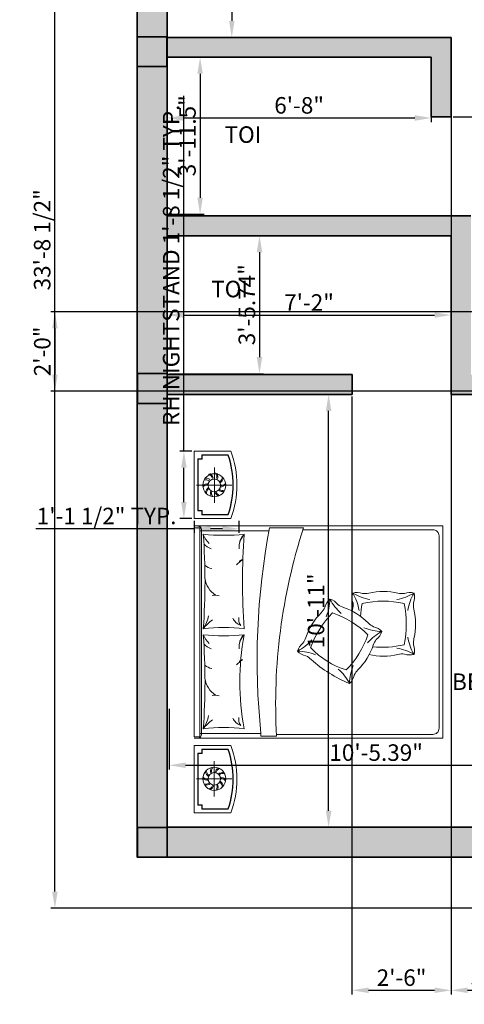
# Model space of a CAD drawing. Units: inches. Extents: x -36 to 490, y -420 to 94.
# Tile 1 of 4: x -36 to 99, y -420 to -122. Entities that reach past the tile are written whole.
import ezdxf

# ---------------------------------------------------------------- set-up
doc = ezdxf.new("R2010")
doc.units = ezdxf.units.IN
for name, color, linetype, lineweight in [('A-ANNO-DIMS', 2, 'Continuous', 18), ('A-AREA-IDEN', 1, 'Continuous', 18), ('A-COLS', 1, 'Continuous', 35), ('A-WALL', 7, 'Continuous', 35), ('furn', 8, 'Continuous', 18)]:
    doc.layers.add(name, color=color, linetype=linetype, lineweight=lineweight)
doc.layers.add('A-WALL-PATT', color=177, linetype='Continuous', lineweight=13, true_color=0x293189)
doc.styles.get("Standard").update_dxf_attribs({"font": 'arial.ttf'})
doc.dimstyles.new('ISO-25', dxfattribs={"dimtxt": 5, "dimasz": 5, "dimexe": 1.25, "dimexo": 0.625, "dimtad": 1, "dimlunit": 3, "dimtxsty": 'Standard', "dimcen": 2.5, "dimadec": 0, "dimazin": 0, "dimtfac": 1, "dimtmove": 0, "dimatfit": 3, "dimfxl": 1, "dimarcsym": 0})

# ---------------------------------------------------------------- blocks, each defined once
blk = doc.blocks.new('*D5')
at = {"layer": 'A-ANNO-DIMS', "color": 0, "lineweight": -2, "transparency": 16777216}
for p, q in [((9.59, -330.42), (9.59, -348.7)), ((134.98, -330.42), (134.98, -348.7)), ((14.59, -347.45), (129.98, -347.45))]:
    blk.add_line(p, q, dxfattribs=at)
at = {"layer": 'A-ANNO-DIMS', "color": 0, "transparency": 16777216}
for points in [[(14.59, -346.62), (14.59, -348.29), (9.59, -347.45)], [(129.98, -346.62), (129.98, -348.29), (134.98, -347.45)]]:
    blk.add_solid(points, dxfattribs=at)
at = {"layer": 'Defpoints', "color": 0, "transparency": 16777216}
for p in [(9.59, -329.79), (134.98, -329.79), (134.98, -347.45)]:
    blk.add_point(p, dxfattribs=at)
at = {"layer": 'A-ANNO-DIMS', "color": 0, "transparency": 16777216, "insert": (72.29, -344.27), "char_height": 5, "attachment_point": 5}
blk.add_mtext('10\'-5.39"', dxfattribs=at)
blk = doc.blocks.new('*D6')
at = {"layer": 'A-ANNO-DIMS', "color": 0, "lineweight": -2, "transparency": 16777216}
for p, q in [((49.72, -235.23), (59.16, -235.23)), ((57.91, -361.23), (57.91, -240.23)), ((49.72, -366.23), (59.16, -366.23))]:
    blk.add_line(p, q, dxfattribs=at)
at = {"layer": 'A-ANNO-DIMS', "color": 0, "transparency": 16777216}
for points in [[(57.07, -240.23), (58.74, -240.23), (57.91, -235.23)], [(57.07, -361.23), (58.74, -361.23), (57.91, -366.23)]]:
    blk.add_solid(points, dxfattribs=at)
at = {"layer": 'Defpoints', "color": 0, "transparency": 16777216}
for p in [(49.09, -235.23), (57.91, -235.23), (49.09, -366.23)]:
    blk.add_point(p, dxfattribs=at)
at = {"layer": 'A-ANNO-DIMS', "color": 0, "transparency": 16777216, "insert": (54.73, -300.73), "char_height": 5, "attachment_point": 5, "rotation": 90}
blk.add_mtext('10\'-11"', dxfattribs=at)
blk = doc.blocks.new('*D7')
at = {"layer": 'A-ANNO-DIMS', "color": 0, "lineweight": -2, "transparency": 16777216}
for p, q in [((8.98, -213.24), (8.98, -209.98)), ((13.98, -211.23), (89.98, -211.23)), ((94.98, -210.6), (94.98, -209.98))]:
    blk.add_line(p, q, dxfattribs=at)
at = {"layer": 'A-ANNO-DIMS', "color": 0, "transparency": 16777216}
for points in [[(13.98, -210.4), (13.98, -212.06), (8.98, -211.23)], [(89.98, -210.4), (89.98, -212.06), (94.98, -211.23)]]:
    blk.add_solid(points, dxfattribs=at)
at = {"layer": 'Defpoints', "color": 0, "transparency": 16777216}
for p in [(94.98, -211.23), (94.98, -211.23), (8.98, -213.87)]:
    blk.add_point(p, dxfattribs=at)
at = {"layer": 'A-ANNO-DIMS', "color": 0, "transparency": 16777216, "insert": (51.98, -208.09), "char_height": 5, "attachment_point": 5}
blk.add_mtext('7\'-2"', dxfattribs=at)
blk = doc.blocks.new('*D8')
at = {"layer": 'A-ANNO-DIMS', "color": 0, "lineweight": -2, "transparency": 16777216}
for p, q in [((9.61, -187.23), (38.23, -187.23)), ((36.98, -192.23), (36.98, -223.97)), ((9.63, -228.97), (38.23, -228.97))]:
    blk.add_line(p, q, dxfattribs=at)
at = {"layer": 'A-ANNO-DIMS', "color": 0, "transparency": 16777216}
for points in [[(36.15, -192.23), (37.82, -192.23), (36.98, -187.23)], [(36.15, -223.97), (37.82, -223.97), (36.98, -228.97)]]:
    blk.add_solid(points, dxfattribs=at)
at = {"layer": 'Defpoints', "color": 0, "transparency": 16777216}
for p in [(8.98, -187.23), (9, -228.97), (36.98, -228.97)]:
    blk.add_point(p, dxfattribs=at)
at = {"layer": 'A-ANNO-DIMS', "color": 0, "transparency": 16777216, "insert": (33.8, -208.1), "char_height": 5, "attachment_point": 5, "rotation": 90}
blk.add_mtext('3\'-5.74"', dxfattribs=at)
blk = doc.blocks.new('*D9')
at = {"layer": 'A-ANNO-DIMS', "color": 0, "lineweight": -2, "transparency": 16777216}
for p, q in [((9.61, -133.23), (20.25, -133.23)), ((19, -138.23), (19, -175.73)), ((9.61, -180.73), (20.25, -180.73))]:
    blk.add_line(p, q, dxfattribs=at)
at = {"layer": 'A-ANNO-DIMS', "color": 0, "transparency": 16777216}
for points in [[(18.16, -138.23), (19.83, -138.23), (19, -133.23)], [(18.16, -175.73), (19.83, -175.73), (19, -180.73)]]:
    blk.add_solid(points, dxfattribs=at)
at = {"layer": 'Defpoints', "color": 0, "transparency": 16777216}
for p in [(8.98, -133.23), (8.98, -180.73), (19, -180.73)]:
    blk.add_point(p, dxfattribs=at)
at = {"layer": 'A-ANNO-DIMS', "color": 0, "transparency": 16777216, "insert": (15.82, -156.98), "char_height": 5, "attachment_point": 5, "rotation": 90}
blk.add_mtext('3\'-11.5"', dxfattribs=at)
blk = doc.blocks.new('*D10')
at = {"layer": 'A-ANNO-DIMS', "color": 0, "lineweight": -2, "transparency": 16777216}
for p, q in [((8.98, -133.85), (8.98, -152.85)), ((88.98, -133.85), (88.98, -152.85)), ((13.98, -151.6), (83.98, -151.6))]:
    blk.add_line(p, q, dxfattribs=at)
at = {"layer": 'A-ANNO-DIMS', "color": 0, "transparency": 16777216}
for points in [[(13.98, -150.77), (13.98, -152.44), (8.98, -151.6)], [(83.98, -150.77), (83.98, -152.44), (88.98, -151.6)]]:
    blk.add_solid(points, dxfattribs=at)
at = {"layer": 'Defpoints', "color": 0, "transparency": 16777216}
for p in [(8.98, -133.23), (88.98, -133.23), (88.98, -151.6)]:
    blk.add_point(p, dxfattribs=at)
at = {"layer": 'A-ANNO-DIMS', "color": 0, "transparency": 16777216, "insert": (48.98, -148.43), "char_height": 5, "attachment_point": 5}
blk.add_mtext('6\'-8"', dxfattribs=at)
blk = doc.blocks.new('*D12')
at = {"layer": 'A-ANNO-DIMS', "color": 0, "lineweight": -2, "transparency": 16777216}
for p, q in [((9.61, 4.77), (29.84, 4.77)), ((28.59, -0.23), (28.59, -122.23)), ((9.61, -127.23), (29.84, -127.23))]:
    blk.add_line(p, q, dxfattribs=at)
at = {"layer": 'A-ANNO-DIMS', "color": 0, "transparency": 16777216}
for points in [[(27.76, -0.23), (29.43, -0.23), (28.59, 4.77)], [(27.76, -122.23), (29.43, -122.23), (28.59, -127.23)]]:
    blk.add_solid(points, dxfattribs=at)
at = {"layer": 'Defpoints', "color": 0, "transparency": 16777216}
for p in [(8.98, 4.77), (8.98, -127.23), (28.59, -127.23)]:
    blk.add_point(p, dxfattribs=at)
at = {"layer": 'A-ANNO-DIMS', "color": 0, "transparency": 16777216, "insert": (25.46, -61.23), "char_height": 5, "attachment_point": 5, "rotation": 90}
blk.add_mtext("11'", dxfattribs=at)
blk = doc.blocks.new('BED-DOUBLE')
for p, q in [((1.11, 73.01), (63.06, 73.01)), ((1.43, 73.57), (1.43, 55.04)), ((62.71, 73.57), (62.71, 52.63))]:
    blk.add_line(p, q)
for points in [[(0, 75.3), (0, 0), (64.18, 0), (64.18, 75.3)], [(63.58, 75.3), (63.58, 73.57), (0.37, 73.57), (0.37, 75.3), (64.18, 75.3)]]:
    blk.add_lwpolyline(points)
for points in [[(2.84, 60.1, 0.058596), (2.84, 72.5, 0.036889), (31.25, 72.5, 0.052163), (31.25, 60.1, 0.093111)], [(33.1, 60.1, 0.058596), (33.1, 72.5, 0.036648), (61.69, 72.5, 0.052163), (61.69, 60.1, 0.036967)], [(0.56, 55.04), (1.43, 55.04, -0.072944), (63.58, 52.45), (63.58, 42.16, 0.092568), (0.56, 50.32)]]:
    blk.add_lwpolyline(points, format="xyb", close=True)
for points in [[(1.11, 50.35), (1.11, 2.97, 0.414214), (2.97, 1.11), (61.21, 1.11, 0.414214), (63.06, 2.97), (63.06, 42.34)], [(25.2, 38.53, 0.091296), (26.33, 43.97, 0.091296), (29.75, 39.6, 0.091296)], [(20.61, 29.25, 0.111006), (31.2, 22.66, 0.119549), (37.88, 33.38, 0.107813), (27.32, 40)], [(27.26, 39.98, 0.121865), (20.61, 29.25, 0.121865)], [(32.26, 18.42, 0.159461), (33.7, 20.96, -0.076283), (34.84, 22.55, 0.115075), (39.49, 30.02, -0.076283), (40.42, 31.75, 0.159461), (42.07, 34.16)], [(36.64, 35.3, 0.091296), (42.07, 34.16, 0.091296), (37.69, 30.75, 0.091296)], [(21.95, 27.08, 0.091296), (16.52, 28.23, 0.091296), (20.9, 31.63, 0.091296)], [(38.64, 25.34, 0.091296), (43.86, 27.24, 0.091296), (41.94, 22.03, 0.091296)], [(43.86, 8.69, 0.159461), (43.73, 11.61, -0.076283), (43.86, 13.56, 0.115075), (43.86, 22.37, -0.076283), (43.73, 24.32, 0.159461), (43.86, 27.24)], [(28.24, 11.72, 0.111006), (40.71, 11.73, 0.119549), (40.71, 24.36, 0.033212), (36.88, 24.95)], [(33.39, 23.85, 0.091296), (32.26, 18.42, 0.091296), (28.84, 22.79)], [(30.52, 10.59, 0.091296), (25.31, 8.69, 0.091296), (27.23, 13.9, 0.091296)], [(41.94, 13.9, 0.091296), (43.86, 8.69, 0.091296), (38.64, 10.59)]]:
    blk.add_lwpolyline(points, format="xyb")
for centre, radius, start, end in [((1.11, 74.12), 1.11, 180, 270), ((9.44, 82.87), 12.28, 237.5379, 257.5233), ((-6.45, 60.91), 14.86, 36.4935, 51.2792), ((18.86, 65.15), 6.88, 96.6849, 148.3182), ((25.81, 69.06), 4.82, 141.8174, 169.8987), ((31.91, 68.38), 5.19, 130.5354, 160.3558), ((35.15, 64), 9.35, 114.6457, 134.1585), ((23.8, 60.91), 14.86, 36.4935, 51.2792), ((39.69, 82.87), 12.28, 237.5379, 257.5233), ((49.11, 65.15), 6.88, 96.6849, 148.3182), ((56.06, 69.06), 4.82, 141.8174, 169.8987), ((62.16, 68.38), 5.19, 130.5354, 160.3558), ((65.4, 64), 9.35, 114.6457, 134.1585), ((63.06, 74.12), 1.11, 270, 0), ((9.94, 68.98), 3.08, 335.8927, 16.1192), ((40.19, 68.98), 3.08, 335.8927, 16.1192), ((7.73, 59.82), 4.12, 114.2916, 160.9896), ((37.98, 59.82), 4.12, 114.2916, 160.9896), ((5.59, 58.96), 2.82, 76.4823, 128.5563), ((11.2, 51.48), 15.49, 36.2085, 45.0849), ((22.66, 60.63), 1.04, 353.7543, 77.2187), ((27.63, 56.56), 5.07, 44.406, 96.8342), ((28.58, 58.33), 3.21, 33.6349, 90.8456), ((35.84, 58.96), 2.82, 76.4823, 128.5563), ((41.46, 51.48), 15.49, 36.2085, 45.0849), ((52.91, 60.63), 1.04, 353.7543, 77.2187), ((57.88, 56.56), 5.07, 44.406, 96.8342), ((58.83, 58.33), 3.21, 33.6349, 90.8456), ((29.5, 40.5), 4.7, 132.4658, 168.7065), ((25.09, 39.6), 4.54, 37.2937, 74.0973), ((32.54, 47.52), 6.44, 233.2983, 250.7472), ((54.12, 12.85), 40.62, 138.3818, 157.7644), ((19.15, 44.34), 6.44, 315.5854, 333.0343), ((24.23, 23.07), 19.38, 45.1307, 71.3884), ((42.4, 41.42), 6.44, 225.7718, 243.2208), ((38.72, 31.4), 4.34, 39.4726, 79.6505), ((19.98, 31.41), 4.7, 222.6522, 258.8929), ((34.58, 8.4), 19.38, 77.0576, 78.7033), ((40.3, 33.58), 6.44, 257.6988, 275.1477), ((42.47, 23.13), 4.34, 71.3996, 111.5774), ((16.17, 21.05), 6.44, 45.7718, 63.2208), ((34.34, 39.4), 19.38, 225.1307, 251.3884), ((44.18, 17.97), 19.38, 166.8711, 193.1289), ((53.75, 18.1), 26.29, 173.1956, 194.0284), ((26.03, 14.95), 6.44, 53.2983, 70.7472), ((34.07, 23.48), 5.38, 218.7754, 250.3571), ((19.02, 12.17), 6.44, 355.0387, 12.4877), ((29.84, 9.96), 4.7, 159.3666, 195.6073), ((26.56, 13.23), 4.7, 254.5791, 290.8198), ((28.81, 2.42), 6.44, 77.6988, 95.1477), ((34.52, 27.6), 19.38, 257.0576, 283.3153), ((40.4, 2.45), 6.44, 85.2252, 102.6741), ((42.71, 13.95), 5.38, 250.7023, 282.284)]:
    blk.add_arc(centre, radius, start, end)
blk = doc.blocks.new('NIGHTSTAND-LAMP-L')
for p, q in [((10.31, 1.49), (10.31, 12.19)), ((4.96, 6.84), (15.66, 6.84))]:
    blk.add_line(p, q)
blk.add_lwpolyline([(0, 1.86), (0, 12.98), (20.4, 12.98), (20.4, 1.86, -0.181818)], format="xyb", close=True)
for points in [[(2.34, 11.87), (2.34, 10.65), (1.11, 10.65)], [(2.45, 11.87), (2.45, 10.54), (1.11, 10.54)], [(2.34, 11.87), (18.07, 11.87)], [(2.34, 11.76), (18.07, 11.76)], [(17.95, 11.87), (17.95, 10.54), (19.29, 10.54)], [(18.07, 11.87), (18.07, 10.65), (19.29, 10.65)]]:
    blk.add_lwpolyline(points)
for points in [[(19.29, 10.65), (19.29, 2.63, -0.167087), (1.11, 2.63), (1.11, 10.65)], [(19.18, 10.65), (19.18, 2.71, -0.165559), (1.22, 2.71), (1.22, 10.65)]]:
    blk.add_lwpolyline(points, format="xyb")
for radius in [3.49, 1.89]:
    blk.add_circle((10.31, 6.84), radius)
for centre, radius, start, end in [((10.62, 9.46), 2.24, 172.17, 218.4897), ((10.4, 9.41), 1.71, 160.3002, 220.538), ((12.1, 8.78), 2.24, 136.17, 182.4897), ((11.89, 8.87), 1.71, 124.3002, 184.538), ((12.89, 7.36), 2.24, 100.17, 146.4897), ((12.78, 7.55), 1.71, 88.3002, 148.538), ((7.89, 7.72), 1.71, 232.3002, 292.538), ((9.02, 9.14), 2.24, 208.17, 254.4897), ((8.87, 8.97), 1.71, 196.3002, 256.538), ((12.7, 5.74), 2.24, 64.17, 110.4897), ((12.72, 5.96), 1.71, 52.3002, 112.538), ((11.74, 4.71), 1.71, 16.3002, 76.538), ((11.59, 4.54), 2.24, 28.17, 74.4897), ((7.91, 7.94), 2.24, 244.17, 290.4897), ((7.84, 6.13), 1.71, 268.3002, 328.538), ((7.72, 6.33), 2.24, 280.17, 326.4897), ((8.72, 4.82), 1.71, 304.3002, 4.538), ((8.52, 4.9), 2.24, 316.17, 2.4897), ((10.22, 4.27), 1.71, 340.3002, 40.538), ((10, 4.22), 2.24, 352.17, 38.4897)]:
    blk.add_arc(centre, radius, start, end)
blk = doc.blocks.new('NIGHTSTAND-LAMP-R')
for p, q in [((10.1, 1.49), (10.1, 12.18)), ((15.45, 6.83), (4.75, 6.83))]:
    blk.add_line(p, q)
blk.add_lwpolyline([(20.4, 1.85), (20.4, 12.98), (0, 12.98), (0, 1.85, 0.181818)], format="xyb", close=True)
for points in [[(2.34, 11.87), (2.34, 10.65), (1.11, 10.65)], [(2.45, 11.87), (2.45, 10.53), (1.11, 10.53)], [(18.07, 11.87), (2.34, 11.87)], [(18.07, 11.76), (2.34, 11.76)], [(17.95, 11.87), (17.95, 10.53), (19.29, 10.53)], [(18.07, 11.87), (18.07, 10.65), (19.29, 10.65)]]:
    blk.add_lwpolyline(points)
for points in [[(1.11, 10.65), (1.11, 2.63, 0.167087), (19.29, 2.63), (19.29, 10.65)], [(1.22, 10.65), (1.22, 2.71, 0.165559), (19.18, 2.71), (19.18, 10.65)]]:
    blk.add_lwpolyline(points, format="xyb")
for radius in [3.49, 1.89]:
    blk.add_circle((10.1, 6.83), radius)
for centre, radius, start, end in [((7.62, 7.54), 1.71, 31.462, 91.6998), ((7.51, 7.35), 2.24, 33.5103, 79.83), ((8.51, 8.86), 1.71, 355.462, 55.6998), ((8.31, 8.77), 2.24, 357.5103, 43.83), ((10.01, 9.4), 1.71, 319.462, 19.6998), ((10.04, 9.55), 2.24, 321.5103, 7.83), ((7.68, 5.95), 1.71, 67.462, 127.6998), ((7.7, 5.73), 2.24, 69.5103, 115.83), ((8.81, 4.54), 2.24, 105.5103, 151.83), ((8.66, 4.7), 1.71, 103.462, 163.6998), ((12.74, 8.03), 2.24, 249.5103, 295.83), ((12.77, 7.81), 1.71, 247.462, 307.6998), ((11.79, 9.06), 1.71, 283.462, 343.6998), ((11.64, 9.23), 2.24, 285.5103, 331.83), ((10.41, 4.22), 2.24, 141.5103, 187.83), ((10.19, 4.27), 1.71, 139.462, 199.6998), ((11.88, 4.9), 2.24, 177.5103, 223.83), ((11.68, 4.81), 1.71, 175.462, 235.6998), ((12.68, 6.32), 2.24, 213.5103, 259.83), ((12.57, 6.13), 1.71, 211.462, 271.6998)]:
    blk.add_arc(centre, radius, start, end)
blk = doc.blocks.new('COLUMN-9X9')
h = blk.add_hatch(color=256)
h.dxf.hatch_style = 1
h.paths.add_polyline_path([(9, 0), (9, 9), (0, 9), (0, 0)])
blk.add_lwpolyline([(0, 9), (9, 9), (9, 0), (0, 0)], close=True)
blk = doc.blocks.new('*D34')
at = {"layer": 'A-ANNO-DIMS', "color": 0, "lineweight": -2, "transparency": 16777216}
for p, q in [((14.1, -252.43), (14.1, -144.93)), ((16.53, -252.43), (12.85, -252.43)), ((14.1, -267.83), (14.1, -257.43)), ((16.53, -272.83), (12.85, -272.83))]:
    blk.add_line(p, q, dxfattribs=at)
at = {"layer": 'A-ANNO-DIMS', "color": 0, "transparency": 16777216}
for points in [[(13.26, -257.43), (14.93, -257.43), (14.1, -252.43)], [(13.26, -267.83), (14.93, -267.83), (14.1, -272.83)]]:
    blk.add_solid(points, dxfattribs=at)
at = {"layer": 'Defpoints', "color": 0, "transparency": 16777216}
for p in [(14.1, -252.43), (17.16, -252.43), (17.16, -272.83)]:
    blk.add_point(p, dxfattribs=at)
at = {"layer": 'A-ANNO-DIMS', "color": 0, "transparency": 16777216, "insert": (10.89, -196.18), "char_height": 5, "attachment_point": 5, "rotation": 90}
blk.add_mtext('RH NIGHTSTAND 1\'-8 1/2" TYP.', dxfattribs=at)
blk = doc.blocks.new('*D35')
at = {"layer": 'A-ANNO-DIMS', "color": 0, "lineweight": -2, "transparency": 16777216}
for p, q in [((17.16, -273.45), (17.16, -277.14)), ((30.76, -273.45), (30.76, -277.14)), ((17.16, -275.89), (-30.75, -275.89)), ((25.76, -275.89), (22.16, -275.89))]:
    blk.add_line(p, q, dxfattribs=at)
at = {"layer": 'A-ANNO-DIMS', "color": 0, "transparency": 16777216}
for points in [[(22.16, -275.06), (22.16, -276.72), (17.16, -275.89)], [(25.76, -275.06), (25.76, -276.72), (30.76, -275.89)]]:
    blk.add_solid(points, dxfattribs=at)
at = {"layer": 'Defpoints', "color": 0, "transparency": 16777216}
for p in [(17.16, -272.83), (30.76, -272.83), (17.16, -275.89)]:
    blk.add_point(p, dxfattribs=at)
at = {"layer": 'A-ANNO-DIMS', "color": 0, "transparency": 16777216, "insert": (-9.3, -272.68), "char_height": 5, "attachment_point": 5}
blk.add_mtext('1\'-1 1/2" TYP.', dxfattribs=at)
blk = doc.blocks.new('*D38')
at = {"layer": 'A-ANNO-DIMS', "color": 0, "lineweight": -2, "transparency": 16777216}
for p, q in [((94.98, -133.85), (94.98, -416.79)), ((133.67, -138.45), (133.67, -416.79)), ((99.98, -415.54), (128.67, -415.54))]:
    blk.add_line(p, q, dxfattribs=at)
at = {"layer": 'A-ANNO-DIMS', "color": 0, "transparency": 16777216}
for points in [[(99.98, -414.7), (99.98, -416.37), (94.98, -415.54)], [(128.67, -414.7), (128.67, -416.37), (133.67, -415.54)]]:
    blk.add_solid(points, dxfattribs=at)
at = {"layer": 'Defpoints', "color": 0, "transparency": 16777216}
for p in [(94.98, -133.23), (133.67, -137.83), (133.67, -415.54)]:
    blk.add_point(p, dxfattribs=at)
at = {"layer": 'A-ANNO-DIMS', "color": 0, "transparency": 16777216, "insert": (114.33, -412.32), "char_height": 5, "attachment_point": 5}
blk.add_mtext('3\'-2 1/2"', dxfattribs=at)
blk = doc.blocks.new('*D41')
at = {"layer": 'A-ANNO-DIMS', "color": 0, "lineweight": -2, "transparency": 16777216}
for p, q in [((326.36, -210.23), (-26.2, -210.23)), ((-24.95, -215.23), (-24.95, -229.23)), ((326.36, -234.23), (-26.2, -234.23))]:
    blk.add_line(p, q, dxfattribs=at)
at = {"layer": 'A-ANNO-DIMS', "color": 0, "transparency": 16777216}
for points in [[(-25.78, -215.23), (-24.12, -215.23), (-24.95, -210.23)], [(-25.78, -229.23), (-24.12, -229.23), (-24.95, -234.23)]]:
    blk.add_solid(points, dxfattribs=at)
at = {"layer": 'Defpoints', "color": 0, "transparency": 16777216}
for p in [(326.98, -210.23), (-24.95, -234.23), (326.98, -234.23)]:
    blk.add_point(p, dxfattribs=at)
at = {"layer": 'A-ANNO-DIMS', "color": 0, "transparency": 16777216, "insert": (-28.13, -222.23), "char_height": 5, "attachment_point": 5, "rotation": 90}
blk.add_mtext('2\'-0"', dxfattribs=at)
blk = doc.blocks.new('*D42')
at = {"layer": 'A-ANNO-DIMS', "color": 0, "lineweight": -2, "transparency": 16777216}
for p, q in [((-0.64, 13.77), (-26.2, 13.77)), ((-24.95, -385.69), (-24.95, 8.77)), ((140.36, -390.69), (-26.2, -390.69))]:
    blk.add_line(p, q, dxfattribs=at)
at = {"layer": 'A-ANNO-DIMS', "color": 0, "transparency": 16777216}
for points in [[(-25.78, 8.77), (-24.12, 8.77), (-24.95, 13.77)], [(-25.78, -385.69), (-24.12, -385.69), (-24.95, -390.69)]]:
    blk.add_solid(points, dxfattribs=at)
at = {"layer": 'Defpoints', "color": 0, "transparency": 16777216}
for p in [(-24.95, 13.77), (-0.02, 13.77), (140.98, -390.69)]:
    blk.add_point(p, dxfattribs=at)
at = {"layer": 'A-ANNO-DIMS', "color": 0, "transparency": 16777216, "insert": (-28.16, -188.46), "char_height": 5, "attachment_point": 5, "rotation": 90}
blk.add_mtext('33\'-8 1/2"', dxfattribs=at)
blk = doc.blocks.new('*D45')
at = {"layer": 'A-ANNO-DIMS', "color": 0, "lineweight": -2, "transparency": 16777216}
for p, q in [((95.61, -151.23), (442.2, -151.23)), ((440.95, -156.23), (440.95, -176.23)), ((101.61, -181.23), (442.2, -181.23))]:
    blk.add_line(p, q, dxfattribs=at)
at = {"layer": 'A-ANNO-DIMS', "color": 0, "transparency": 16777216}
for points in [[(440.11, -156.23), (441.78, -156.23), (440.95, -151.23)], [(440.11, -176.23), (441.78, -176.23), (440.95, -181.23)]]:
    blk.add_solid(points, dxfattribs=at)
at = {"layer": 'Defpoints', "color": 0, "transparency": 16777216}
for p in [(94.98, -151.23), (100.98, -181.23), (440.95, -181.23)]:
    blk.add_point(p, dxfattribs=at)
at = {"layer": 'A-ANNO-DIMS', "color": 0, "transparency": 16777216, "insert": (437.77, -166.23), "char_height": 5, "attachment_point": 5, "rotation": 90}
blk.add_mtext('2\'-6"', dxfattribs=at)
blk = doc.blocks.new('*D46')
at = {"layer": 'A-ANNO-DIMS', "color": 0, "lineweight": -2, "transparency": 16777216}
for p, q in [((64.98, -235.85), (64.98, -416.79)), ((94.98, -235.85), (94.98, -416.79)), ((69.98, -415.54), (89.98, -415.54))]:
    blk.add_line(p, q, dxfattribs=at)
at = {"layer": 'A-ANNO-DIMS', "color": 0, "transparency": 16777216}
for points in [[(69.98, -414.7), (69.98, -416.37), (64.98, -415.54)], [(89.98, -414.7), (89.98, -416.37), (94.98, -415.54)]]:
    blk.add_solid(points, dxfattribs=at)
at = {"layer": 'Defpoints', "color": 0, "transparency": 16777216}
for p in [(64.98, -235.23), (94.98, -235.23), (94.98, -415.54)]:
    blk.add_point(p, dxfattribs=at)
at = {"layer": 'A-ANNO-DIMS', "color": 0, "transparency": 16777216, "insert": (79.98, -412.36), "char_height": 5, "attachment_point": 5}
blk.add_mtext('2\'-6"', dxfattribs=at)

msp = doc.modelspace()

# ---------------------------------------------------------------- hatches: boundary and pattern name
at = {"layer": 'A-WALL-PATT'}
h = msp.add_hatch(color=256, dxfattribs=at)
h.dxf.hatch_style = 1
h.paths.add_polyline_path([(132.114, 13.772), (8.901, 13.772), (8.901, 4.772), (132.114, 4.772)])
h.paths.add_polyline_path([(274.98, 13.772), (141.114, 13.772), (141.114, 4.772), (274.98, 4.772)])
h.paths.add_polyline_path([(407.097, 13.772), (283.98, 13.772), (283.98, 4.772), (407.097, 4.772)])
h.paths.add_polyline_path([(280.984, 4.772), (274.984, 4.772), (274.984, -127.228), (280.984, -127.228)])
h.paths.add_polyline_path([(274.984, -127.228), (176.984, -127.228), (176.984, -133.228), (274.984, -133.228)])
h.paths.add_polyline_path([(140.984, 4.772), (134.984, 4.772), (134.984, -128.829), (140.984, -128.829)])
h.paths.add_polyline_path([(8.984, 4.772), (8.901, 4.772), (-0.016, 4.772), (-0.016, -127.003), (8.984, -127.003)])
h.paths.add_polyline_path([(94.984, -127.228), (8.984, -127.228), (8.984, -133.228), (88.984, -133.228), (88.984, -151.228), (94.984, -151.228), (94.984, -133.228)])
h.paths.add_polyline_path([(8.984, -136.003), (-0.016, -136.003), (-0.016, -228.965), (8.984, -228.965)])
h.paths.add_polyline_path([(100.984, -181.228), (98.984, -181.228), (88.984, -181.228), (8.984, -181.228), (8.984, -187.228), (88.984, -187.228), (94.984, -187.228), (94.984, -235.228), (134.793, -235.228), (134.793, -229.228), (100.984, -229.228)])
h.paths.add_polyline_path([(64.984, -229.228), (9.003, -229.228), (9.003, -235.228), (64.984, -235.228)], flags=17)
h.paths.add_polyline_path([(8.984, -237.965), (-0.016, -237.965), (-0.016, -366.285), (8.984, -366.285)])
h.paths.add_polyline_path([(132.054, -366.228), (9.018, -366.228), (9.018, -375.228), (132.054, -375.228)])
h.paths.add_polyline_path([(140.984, -271.228), (134.984, -271.228), (134.984, -366.131), (140.984, -366.131)])

# ---------------------------------------------------------------- linework, layer by layer
at = {"layer": 'A-WALL'}
for p, q in [((8.984, -366.228), (8.984, 4.772)), ((8.984, -127.228), (94.984, -127.228)), ((94.984, -133.228), (94.984, -127.228)), ((8.984, -133.228), (88.984, -133.228)), ((88.984, -133.228), (88.984, -151.228)), ((94.984, -133.228), (94.984, -151.228)), ((88.984, -151.228), (94.984, -151.228)), ((88.984, -181.228), (8.984, -181.228)), ((88.984, -181.228), (98.984, -181.228)), ((98.984, -181.228), (100.984, -181.228)), ((88.984, -187.228), (8.984, -187.228)), ((88.984, -187.228), (94.984, -187.228)), ((94.984, -187.228), (94.984, -235.228)), ((64.984, -229.228), (8.984, -229.228)), ((64.984, -235.228), (64.984, -229.228)), ((64.984, -235.228), (8.984, -235.228)), ((94.984, -235.228), (134.984, -235.228)), ((140.984, -366.228), (8.984, -366.228))]:
    msp.add_line(p, q, dxfattribs=at)
msp.add_lwpolyline([(-0.016, 13.772), (415.984, 13.772), (415.984, -375.228), (-0.016, -375.228)], close=True, dxfattribs=at)

# ---------------------------------------------------------------- block references
at = {"layer": 'A-COLS'}
for p, rotation in [((-0.073, -127.003), 269.9999999999998), ((0.002, -228.965), 269.9999999999997), ((0.018, -366.285), 269.9999999999997)]:
    msp.add_blockref('COLUMN-9X9', p, dxfattribs=dict(at, rotation=rotation))
at = {"layer": 'furn'}
for name, p, rotation in [('NIGHTSTAND-LAMP-R', (30.14, -272.829), 89.99999999999969), ('BED-DOUBLE', (92.46, -339.23), 90.00000000000017), ('NIGHTSTAND-LAMP-L', (30.145, -361.858), 89.99999999999939)]:
    msp.add_blockref(name, p, dxfattribs=dict(at, rotation=rotation))

# ---------------------------------------------------------------- texts
at = {"layer": 'A-AREA-IDEN', "char_height": 5, "attachment_point": 1}
for s, width, insert in [('{TOI}', 49.01082, (26.402, -154.131)), ('{TOI}', 39.56837, (22.355, -200.857)), ('{BEDROOM}', 15.30121, (95.268, -319.675))]:
    msp.add_mtext_dynamic_manual_height_columns(s, width=width, gutter_width=12.5, heights=[0], dxfattribs=dict(at, insert=insert))

# ---------------------------------------------------------------- dimensions: what is measured, and where the dimension line sits
at = {"layer": 'A-ANNO-DIMS'}
for base, p1, p2, override, picture, middle in [((-24.949, 13.772), (140.984, -390.685), (-0.016, 13.772), {"dimdec": 1, "dimlfac": 1, "dimrnd": 0, "dimzin": 1, "dimdsep": 46, "dimlunit": 4, "dimfrac": 2}, '*D42', (-28.161, -188.457)), ((28.594, -127.228), (8.984, 4.772), (8.984, -127.228), {"dimclrd": 0, "dimclre": 0, "dimclrt": 0}, '*D12', (25.459, -61.228)), ((18.997, -180.728), (8.984, -133.228), (8.984, -180.728), {"dimclrd": 0, "dimclre": 0, "dimclrt": 0}, '*D9', (15.818, -156.978)), ((440.947, -181.228), (94.984, -151.228), (100.984, -181.228), {"dimdec": 1, "dimlfac": 1, "dimrnd": 0, "dimzin": 1, "dimdsep": 46, "dimlunit": 4, "dimfrac": 2}, '*D45', (437.769, -166.228)), ((36.984, -228.965), (8.984, -187.228), (9.003, -228.965), {"dimclrd": 0, "dimclre": 0, "dimclrt": 0}, '*D8', (33.805, -208.097)), ((-24.949, -234.228), (326.984, -210.228), (326.984, -234.228), {"dimdec": 1, "dimlfac": 1, "dimrnd": 0, "dimzin": 1, "dimdsep": 46, "dimlunit": 4, "dimfrac": 2}, '*D41', (-28.126, -222.228)), ((57.906, -235.228), (49.094, -366.228), (49.094, -235.228), {"dimclrd": 0, "dimclre": 0, "dimclrt": 0}, '*D6', (54.729, -300.728))]:
    dim = msp.add_linear_dim(base=base, p1=p1, p2=p2, angle=90, dimstyle='ISO-25', override=override, dxfattribs=at)
    dim.commit()
    dim.dimension.update_dxf_attribs({"geometry": picture, "text_midpoint": middle})
for base, p1, p2, override, picture, middle in [((88.984, -151.604), (8.984, -133.228), (88.984, -133.228), {"dimclrd": 0, "dimclre": 0, "dimclrt": 0}, '*D10', (48.984, -148.426)), ((133.675, -415.535), (94.984, -133.228), (133.675, -137.829), {"dimdec": 1, "dimlfac": 1, "dimrnd": 0, "dimzin": 1, "dimdsep": 46, "dimlunit": 4, "dimfrac": 2}, '*D38', (114.33, -412.323)), ((94.984, -211.228), (8.984, -213.868), (94.984, -211.228), {"dimclrd": 0, "dimclre": 0, "dimclrt": 0}, '*D7', (51.984, -208.093)), ((94.984, -415.535), (64.984, -235.228), (94.984, -235.228), {"dimdec": 1, "dimlfac": 1, "dimrnd": 0, "dimzin": 1, "dimdsep": 46, "dimlunit": 4, "dimfrac": 2}, '*D46', (79.984, -412.357)), ((134.984, -347.452), (9.595, -329.792), (134.984, -329.792), {"dimclrd": 0, "dimclre": 0, "dimclrt": 0}, '*D5', (72.289, -344.273))]:
    dim = msp.add_linear_dim(base=base, p1=p1, p2=p2, dimstyle='ISO-25', override=override, dxfattribs=at)
    dim.commit()
    dim.dimension.update_dxf_attribs({"geometry": picture, "text_midpoint": middle})
for base, p1, p2, angle, text, picture, middle in [((14.096, -252.426), (17.157, -272.829), (17.157, -252.426), 90, 'RH NIGHTSTAND <> TYP.', '*D34', (10.886, -196.181)), ((17.157, -275.889), (30.758, -272.829), (17.157, -272.829), 180, '<> TYP.', '*D35', (-9.297, -272.679))]:
    dim = msp.add_linear_dim(base=base, p1=p1, p2=p2, angle=angle, text=text, dimstyle='ISO-25', override={"dimdec": 1, "dimlfac": 1, "dimrnd": 0, "dimzin": 1, "dimdsep": 46, "dimlunit": 4, "dimfrac": 2}, dxfattribs=at)
    dim.commit()
    dim.dimension.update_dxf_attribs({"geometry": picture, "text_midpoint": middle})

doc.saveas('drawing.dxf')
